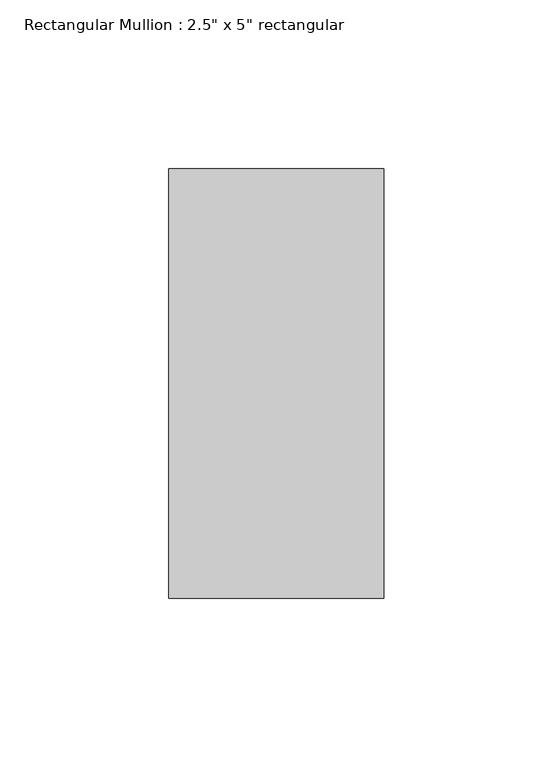
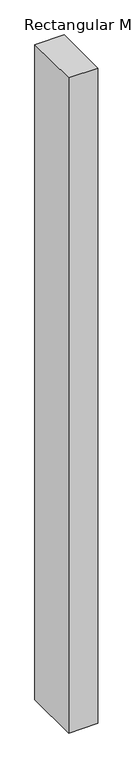
"""IFC4 building model written with IfcOpenShell, lengths in millimetres: member geometry."""

from ifc_helpers import new_model, si_unit, frame, origin, place, context, project, spatial, polyline, outline, extrude, source, transform, mapped, element, save


def member_a0c6f7ef(model_context):
    return source(origin(), model_context, "Body", "SweptSolid", [
        extrude(outline(polyline([(0.0, 63.5), (0.0, -63.5), (-63.5, -63.5), (-63.5, 63.5), (0.0, 63.5)])), frame((0.0, 0.0, -1510.5980535), z_axis=(0.0, 0.0, 1.0), x_axis=(1.0, 0.0, 0.0)), (0.0, 0.0, 1.0), 1510.5980535),
    ])


if __name__ == "__main__":
    model = new_model("IFC4")
    model_context = context("Model", 3, world=origin())
    ifc_project = project(units=[si_unit("LENGTHUNIT", "METRE", prefix="MILLI")], contexts=[model_context])
    site = spatial("IfcSite", under=ifc_project)
    building = spatial("IfcBuilding", under=site)
    placement = place(None, origin())
    member_shape = member_a0c6f7ef(model_context)
    element("IfcMember", 1, ObjectType="Rectangular Mullion : 2.5\" x 5\" rectangular", at=placement, inside=building, context=model_context, shape_type="MappedRepresentation", body=[
        mapped(member_shape, transform((0.0, 0.0, 0.0), x_axis=(1.0, 0.0, 0.0), y_axis=(0.0, 1.0, 0.0), z_axis=(0.0, 0.0, 1.0))),
    ])
    save(model, "model.ifc")

# Revit data of these elements
# Type "Rectangular Mullion : 2.5\" x 5\" rectangular"
#   built-in parameter 1007304 = 0.416667 (stored number, unit not read)
#   built-in parameter 1007301 = 0.104167 (stored number, unit not read)
#   built-in parameter 1007300 = 0.104167 (stored number, unit not read)
# Element 1 (IfcMember, "Rectangular Mullion : 2.5\" x 5\" rectangular")
#   Materials on its faces: "Aluminum"
# Materials
#   "Aluminum": class "Metal", colour RGB 247 247 247, transparency 0, Description = "Aluminum 6061", Cost = 0
